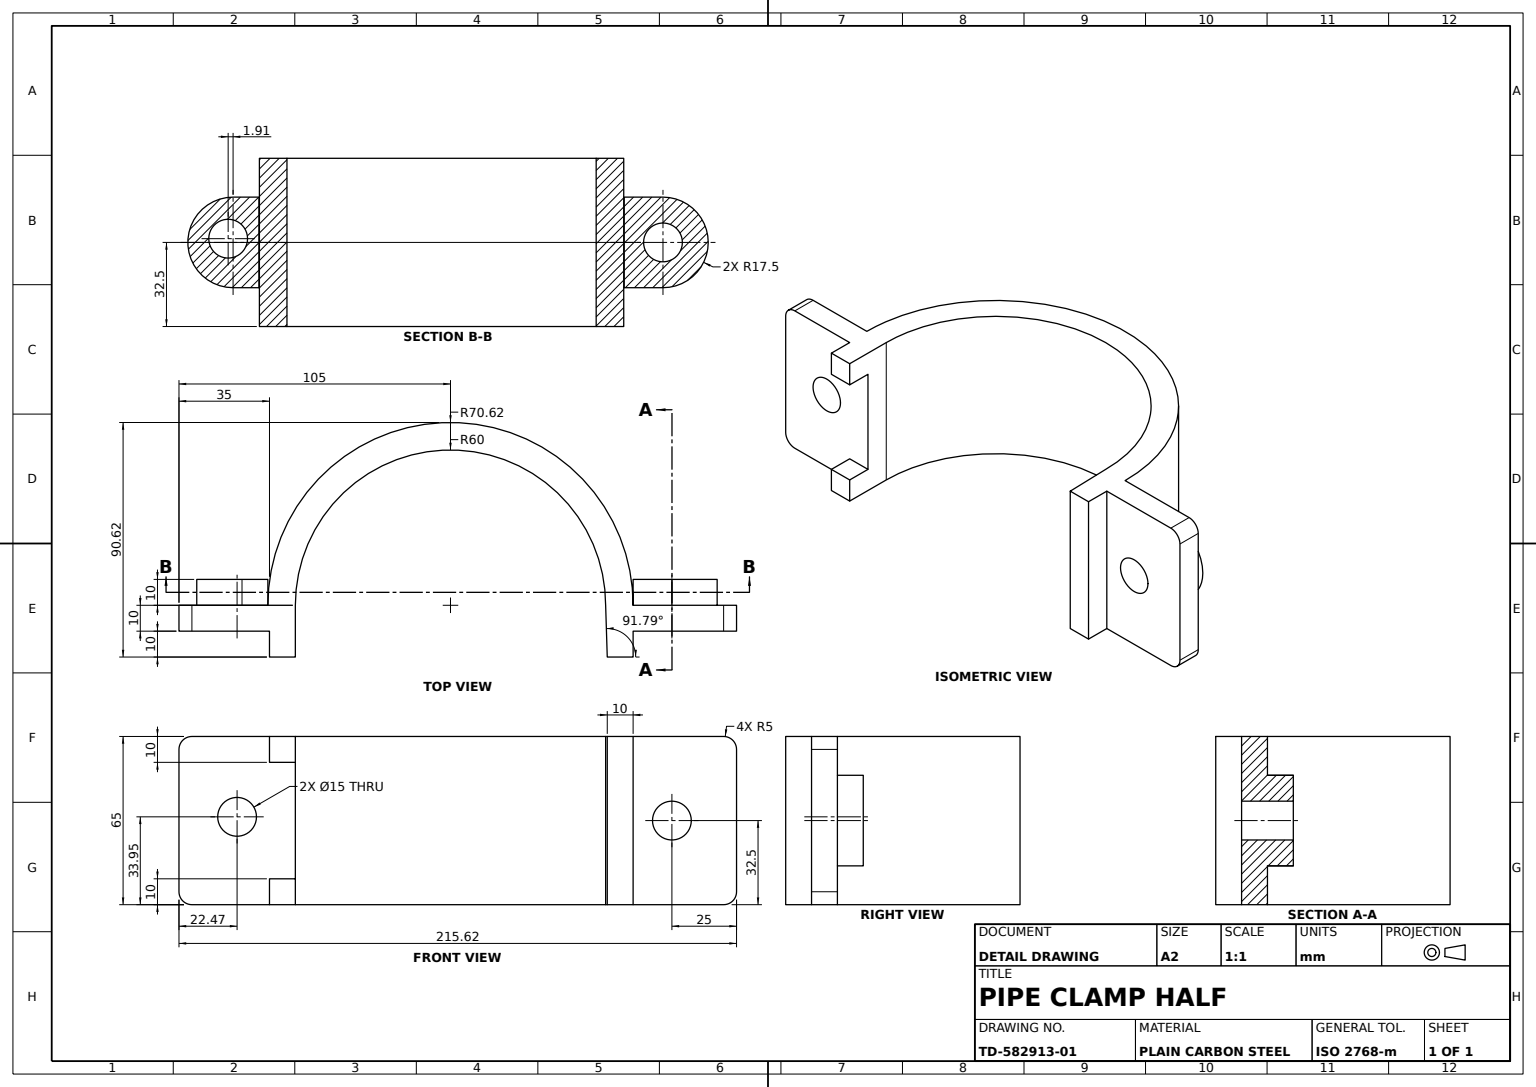
SolidWorks part; units mm, degrees
material "Plain Carbon Steel"
ref_plane "Front Plane" through (0, 0, 0) normal (0, 0, 1) x (1, 0, 0)
ref_plane "Top Plane" through (0, 0, 0) normal (0, 1, 0) x (1, 0, 0)
ref_plane "Right Plane" through (0, 0, 0) normal (1, 0, 0) x (0, 0, -1)
sketch "Flange Step A Sketch" plane through (0, 0, 0) normal (0, 0, 1) x (1, 0, 0)
  line L1 (0, 10) -> (-40, 10)
  line L2 (-45, 70) -> (-45, 15)
  line L4 (0, 75) -> (-40, 75)
  line L8 (0, 75) -> (0, 10)
  arc A0 (-45, 15) -> (-40, 10) centre (-40, 15) ccw
  arc A1 (-40, 75) -> (-45, 70) centre (-40, 70) ccw
  dimension "D1" = 10
  dimension "D2" = 10
  dimension "D3" = 5
  dimension "D4" = 40
  dimension "D5" = 65
  dimension "D6" = 10
extrude "Flange Step A" add sketch "Flange Step A Sketch" along normal blind 10
sketch "Flange Rib Sketch" plane through (0, 0, 10) normal (0, 0, 1) x (1, 0, 0)
  line L0 (0, 75) -> (-10, 75)
  line L1 (0, 75) -> (-40, 75) construction
  line L2 (-10, 75) -> (-10, 65)
  line L3 (-10, 65) -> (0, 65)
  line L4 (0, 10) -> (0, 75) construction
  line L5 (0, 65) -> (0, 75)
  line L6 (0, 10) -> (0, 20)
  line L7 (0, 20) -> (-10, 20)
  line L8 (-10, 20) -> (-10, 10)
  line L9 (-40, 10) -> (0, 10) construction
  line L10 (-10, 10) -> (0, 10)
  dimension "D1" = 10
extrude "Flange Rib" add sketch "Flange Rib Sketch" along normal blind 10
sketch "Clamp Band Sketch" plane through (0, 75, 0) normal (0, 1, 0) x (1, 0, 0)
  line L1 (-40, -10) -> (-40, 0) construction
  line L2 (0, 0) -> (120, 0)
  line L5 (-10.6241, 0) -> (0, 0)
  line L6 (120, 0) -> (130.6241, 0)
  line L7 (119.1608, -10) -> (120, -10)
  arc A0 (120, 0) -> (0, 0) centre (60, 0) ccw
  arc A1 (130.6241, 0) -> (-10.6241, 0) centre (60, 0) ccw
  line M1 (0, 0) -> (-40, 0)
  dimension "D1" = 120
  dimension "D2" = 141.2482
  dimension "D3" = 60
  dimension "D4" = 70.6241
  dimension "D5" = 159.1608
extrude "Clamp Band" add sketch "Clamp Band Sketch" against normal blind 65 contours L6 A1 A0 M1
sketch "Flange Step B Sketch" plane through (0, 0, 0) normal (0, 0, 1) x (1, 0, 0)
  line L0 (130.6241, 75) -> (165.6241, 75)
  line L3 (130.6241, 10) -> (165.6241, 10)
  line L6 (120, 10) -> (120, 75) construction
  line L7 (170.6241, 70) -> (170.6241, 15)
  line L8 (130.6241, 75) -> (130.6241, 10)
  arc A0 (170.6241, 70) -> (165.6241, 75) centre (165.6241, 70) ccw
  arc A1 (165.6241, 10) -> (170.6241, 15) centre (165.6241, 15) ccw
  dimension "D1" = 10
  dimension "D2" = 10
  dimension "D3" = 5
  dimension "D4" = 50.6241
extrude "Flange Step B" add sketch "Flange Step B Sketch" along normal blind 10 separate body
sketch "Flange Web Sketch" plane through (0, 75, 0) normal (0, 1, 0) x (1, 0, 0)
  line L0 (130.6241, 0) -> (130.6241, -20)
  line L1 (130.6241, -20) -> (120.6241, -20)
  line L2 (120.6241, -20) -> (120, 0)
  line L3 (120, 0) -> (130.6241, 0)
  line L4 (0, -20) -> (0, 0) construction
  line L5 (-10.6241, 0) -> (-40, 0) construction
  dimension "D1" = 120.6241
  dimension "D2" = 20
extrude "Flange Web" add sketch "Flange Web Sketch" against normal blind 65
sketch "Mounting Lug 1 Sketch" plane through (0, 0, 0) normal (0, 0, -1) x (-1, 0, 0)
  line L0 (-165.6241, 75) -> (-130.6241, 75) construction
  line L1 (-130.6241, 60) -> (-145.6241, 60)
  line L2 (-130.6241, 10) -> (-130.6241, 75) construction
  line L4 (-130.6241, 25) -> (-145.6241, 25)
  line L5 (-130.6241, 60) -> (-130.6241, 25)
  arc A0 (-145.6241, 60) -> (-145.6241, 25) centre (-145.6241, 42.5) ccw
  dimension "D1" = 35
  dimension "D2" = 17.5
  dimension "D3" = 15
  dimension "D4" = 32.5
extrude "Mounting Lug 1" add sketch "Mounting Lug 1 Sketch" along normal blind 10
sketch "Mounting Lug 2 Sketch" plane through (0, 0, 0) normal (0, 0, -1) x (-1, 0, 0)
  line L0 (10.6241, 60) -> (10.6241, 25)
  line L1 (10.6241, 10) -> (10.6241, 75) construction
  line L2 (40, 10) -> (10.6241, 10) construction
  line L3 (10.6241, 60) -> (20.6241, 60)
  line L5 (20.6241, 25) -> (10.6241, 25)
  arc A0 (20.6241, 25) -> (20.6241, 60) centre (20.6241, 42.5) ccw
  dimension "D1" = 35
  dimension "D2" = 17.5
  dimension "D3" = 10
  dimension "D4" = 32.5
extrude "Mounting Lug 2" add sketch "Mounting Lug 2 Sketch" along normal blind 10
sketch "Bolt Hole 1 Sketch" plane through (0, 0, -10) normal (0, 0, -1) x (-1, 0, 0)
  circle A0 centre (-145.6241, 42.5) radius 7.5
  dimension "D1" = 15
  dimension "D2" = 15
extrude "Bolt Hole 1 Ø15" cut sketch "Bolt Hole 1 Sketch" against normal blind 20
sketch "Bolt Hole 2 Sketch" plane through (0, 0, -10) normal (0, 0, -1) x (-1, 0, 0)
  line L0 (10.6241, 60) -> (10.6241, 25) construction
  line L1 (20.6241, 60) -> (10.6241, 60) construction
  circle A0 centre (22.5308, 43.9465) radius 7.5
  dimension "D1" = 15
  dimension "D2" = 15
  dimension "D3" = 11.9067
  dimension "D4" = 16.0535
extrude "Bolt Hole 2 Ø15" cut sketch "Bolt Hole 2 Sketch" against normal blind 20
